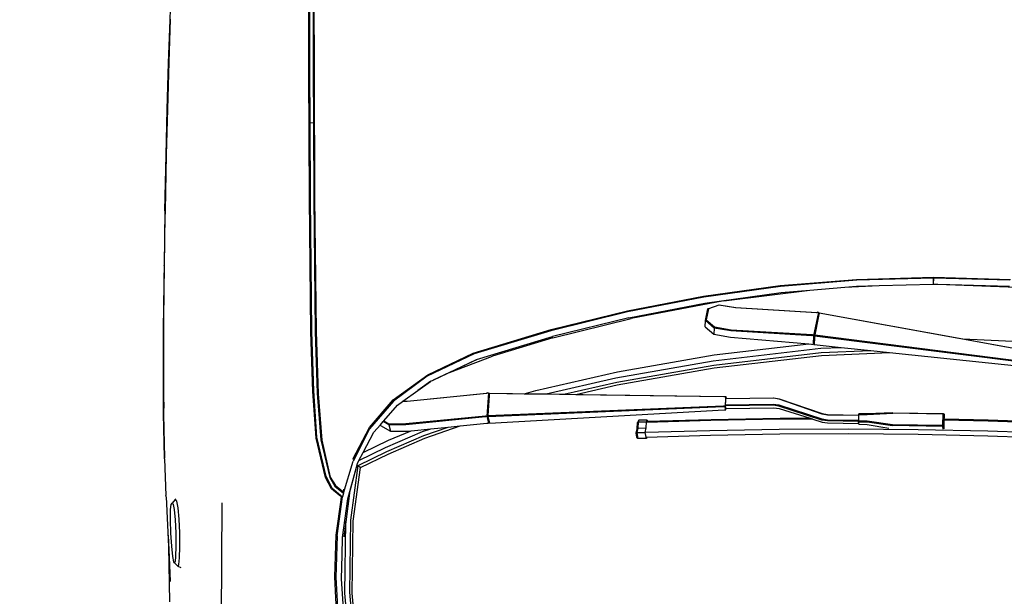
# Model space of a CAD drawing. Units: inches. Extents: x 0 to 4258, y 0 to 3769.
# Tile 12 of 30: x 3726 to 3763, y 3082 to 3104. Entities that reach past the tile are written whole.
import ezdxf

# ---------------------------------------------------------------- set-up
doc = ezdxf.new("R2010")
doc.units = ezdxf.units.IN
doc.header["$MEASUREMENT"] = 0
doc.layers.get('0').update_dxf_attribs({"color": 16})
doc.layers.add('A-ANNO-DIMS', color=250, linetype='Continuous', lineweight=18)
doc.layers.add('C-PKNG-VEHI', color=8, linetype='Continuous', lineweight=18)
doc.layers.add('Edges', color=250, linetype='Continuous')
doc.styles.get("Standard").update_dxf_attribs({"font": 'arial.ttf'})
doc.dimstyles.get("Standard").update_dxf_attribs({"dimtxt": 7, "dimasz": 0.18, "dimexe": 0.18, "dimexo": 0.0625, "dimgap": 0.09, "dimtad": 0, "dimtih": 1, "dimtoh": 1, "dimzin": 0, "dimdsep": 46, "dimlunit": 3, "dimtxsty": 'Standard', "dimcen": 0.09, "dimadec": 0, "dimazin": 0, "dimtfac": 1, "dimtofl": 0, "dimtmove": 0, "dimatfit": 3, "dimfxl": 1, "dimtolj": 1, "dimtzin": 0, "dimarcsym": 0})

# ---------------------------------------------------------------- blocks, each defined once
blk = doc.blocks.new('Nissan Qashqai pl')
at = {"layer": 'Edges'}
for p, q in [((8.4387, 12.0674), (8.4359, 11.9861)), ((8.4397, 12.0674), (8.4369, 11.9861)), ((8.4517, 12.0674), (8.4489, 11.9858)), ((8.4541, 11.9857), (8.4568, 12.0669)), ((8.3575, 12.0475), (8.3104, 11.7881)), ((8.3406, 11.9567), (8.3448, 12.0536)), ((8.3565, 11.8707), (8.3746, 12.0435)), ((8.336, 11.7828), (8.3688, 12.0419)), ((8.3702, 12.0427), (8.3374, 11.7826)), ((8.2765, 11.9273), (8.2804, 12.0305)), ((8.2682, 11.9221), (8.2708, 12.0123)), ((8.2719, 12.0118), (8.2695, 11.9221)), ((8.2765, 11.9273), (8.2788, 12.0114)), ((8.3406, 11.9567), (8.3495, 12.0053)), ((8.4359, 11.9861), (8.4348, 11.9346)), ((8.4369, 11.9861), (8.4358, 11.9346)), ((8.4489, 11.9858), (8.4471, 11.9043)), ((8.4523, 11.9043), (8.4541, 11.9857)), ((8.31, 11.7882), (8.3406, 11.9567)), ((8.4272, 11.8746), (8.4281, 11.9336)), ((8.4287, 11.9335), (8.4278, 11.8745)), ((8.4281, 11.9336), (8.429, 11.9345)), ((8.4281, 11.9336), (8.4287, 11.9336)), ((8.4287, 11.9335), (8.4281, 11.9336)), ((8.429, 11.9345), (8.4287, 11.9336)), ((8.4287, 11.9336), (8.4287, 11.9335)), ((8.4418, 11.9332), (8.4287, 11.9335)), ((8.4328, 11.9347), (8.429, 11.9345)), ((8.429, 11.9345), (8.4326, 11.9345)), ((8.4328, 11.9347), (8.4326, 11.9345)), ((8.4326, 11.9345), (8.4348, 11.9344)), ((8.4348, 11.9346), (8.4328, 11.9347)), ((8.4348, 11.9346), (8.4348, 11.9344)), ((8.4358, 11.9346), (8.4348, 11.9346)), ((8.4348, 11.9344), (8.4358, 11.9344)), ((8.4358, 11.9346), (8.4358, 11.9344)), ((8.4459, 11.9344), (8.4358, 11.9346)), ((8.4358, 11.9344), (8.4422, 11.9342)), ((8.441, 11.8742), (8.4418, 11.9332)), ((8.4418, 11.9332), (8.4422, 11.9342)), ((8.4431, 11.9332), (8.4418, 11.9332)), ((8.4422, 11.9342), (8.4459, 11.9344)), ((8.4422, 11.9342), (8.4431, 11.9332)), ((8.4431, 11.9332), (8.4422, 11.8742)), ((8.4464, 11.9334), (8.4431, 11.9332)), ((8.4459, 11.9344), (8.4459, 11.9344)), ((8.2708, 11.8319), (8.2682, 11.9221)), ((8.2763, 11.9223), (8.2695, 11.9221)), ((8.2695, 11.9221), (8.2763, 11.9219)), ((8.2695, 11.9221), (8.2719, 11.8323)), ((8.2763, 11.9223), (8.2764, 11.9263)), ((8.2763, 11.9219), (8.2763, 11.9223)), ((8.2781, 11.8585), (8.2763, 11.9219)), ((8.2764, 11.9263), (8.2765, 11.9273)), ((8.4471, 11.9043), (8.4464, 11.8227)), ((8.4516, 11.823), (8.4523, 11.9043)), ((8.3542, 11.8485), (8.3565, 11.8707)), ((8.3599, 11.7906), (8.3565, 11.8707)), ((8.4272, 11.8746), (8.4286, 11.8445)), ((8.4292, 11.8445), (8.4278, 11.8745)), ((8.4368, 11.8443), (8.441, 11.8742)), ((8.438, 11.8443), (8.4422, 11.8742)), ((8.28, 11.818), (8.2781, 11.8585)), ((8.2788, 11.8327), (8.2781, 11.8585)), ((8.2789, 11.8319), (8.2781, 11.8585)), ((8.4408, 11.8444), (8.4452, 11.8698)), ((8.3505, 11.8139), (8.3542, 11.8485)), ((8.3567, 11.7903), (8.3542, 11.8485)), ((8.4286, 11.8445), (8.4285, 11.8345)), ((8.4291, 11.8345), (8.4292, 11.8445)), ((8.4366, 11.8345), (8.4368, 11.8443)), ((8.4379, 11.8345), (8.438, 11.8443)), ((8.4406, 11.8344), (8.4408, 11.8444)), ((8.2781, 11.7423), (8.2708, 11.8319)), ((8.2719, 11.8323), (8.2793, 11.7426)), ((8.2789, 11.8319), (8.2788, 11.8327)), ((8.28, 11.818), (8.2789, 11.8319)), ((8.4291, 11.8345), (8.4285, 11.8345)), ((8.4298, 11.8345), (8.4291, 11.8345)), ((8.4292, 11.7978), (8.4298, 11.8345)), ((8.4304, 11.8345), (8.4298, 11.7978)), ((8.4304, 11.8345), (8.4298, 11.8345)), ((8.436, 11.8344), (8.4304, 11.8345)), ((8.4355, 11.7977), (8.436, 11.8344)), ((8.4366, 11.8343), (8.436, 11.8344)), ((8.4366, 11.8345), (8.4379, 11.8345)), ((8.4366, 11.8344), (8.4366, 11.8345)), ((8.4373, 11.8344), (8.4366, 11.8344)), ((8.4373, 11.8344), (8.4366, 11.8343)), ((8.4366, 11.8343), (8.4366, 11.8344)), ((8.4373, 11.8344), (8.4367, 11.7977)), ((8.4379, 11.8344), (8.4373, 11.8344)), ((8.4379, 11.8343), (8.4373, 11.8344)), ((8.4379, 11.8344), (8.4379, 11.8345)), ((8.4397, 11.8344), (8.4379, 11.8343)), ((8.4379, 11.8343), (8.4379, 11.8344)), ((8.4391, 11.7978), (8.4397, 11.8344)), ((8.4406, 11.8344), (8.4397, 11.8344)), ((8.2834, 11.7773), (8.28, 11.818)), ((8.3472, 11.7821), (8.3505, 11.8139)), ((8.3516, 11.79), (8.3505, 11.8139)), ((8.4464, 11.8227), (8.4468, 11.7413)), ((8.452, 11.7418), (8.4516, 11.823)), ((8.3662, 11.6639), (8.3516, 11.79)), ((8.3713, 11.6645), (8.3567, 11.7903)), ((8.3745, 11.665), (8.3599, 11.7906)), ((8.4107, 11.7411), (8.4281, 11.7914)), ((8.4287, 11.7914), (8.4111, 11.741)), ((8.4179, 11.7406), (8.4344, 11.7912)), ((8.4357, 11.7912), (8.4193, 11.7407)), ((8.4281, 11.7914), (8.4292, 11.7978)), ((8.4298, 11.7978), (8.4287, 11.7914)), ((8.4344, 11.7912), (8.4355, 11.7977)), ((8.4347, 11.7805), (8.4381, 11.7914)), ((8.4367, 11.7977), (8.4357, 11.7912)), ((8.4381, 11.7914), (8.4391, 11.7978)), ((8.3038, 11.6903), (8.3095, 11.7853)), ((8.3099, 11.7851), (8.3042, 11.6901)), ((8.3092, 11.7863), (8.3093, 11.7873)), ((8.3092, 11.7863), (8.3099, 11.7851)), ((8.3095, 11.7853), (8.3092, 11.7863)), ((8.3093, 11.7873), (8.3367, 11.7816)), ((8.3159, 11.7869), (8.3093, 11.7873)), ((8.31, 11.7882), (8.3104, 11.7881)), ((8.3104, 11.7881), (8.3159, 11.7869)), ((8.3159, 11.7869), (8.336, 11.7828)), ((8.3298, 11.6848), (8.3355, 11.7798)), ((8.3369, 11.7796), (8.3312, 11.6846)), ((8.3355, 11.7798), (8.3366, 11.7806)), ((8.336, 11.7828), (8.3374, 11.7826)), ((8.3367, 11.7816), (8.3366, 11.7806)), ((8.3366, 11.7806), (8.3369, 11.7796)), ((8.3367, 11.7816), (8.347, 11.7811)), ((8.3374, 11.7826), (8.3406, 11.7824)), ((8.3458, 11.7813), (8.3406, 11.7824)), ((8.3406, 11.7824), (8.3457, 11.7821)), ((8.3458, 11.7813), (8.3457, 11.7821)), ((8.3457, 11.7821), (8.3472, 11.7821)), ((8.347, 11.7811), (8.3458, 11.7813)), ((8.3464, 11.7761), (8.3467, 11.7791)), ((8.3467, 11.7791), (8.347, 11.7811)), ((8.4337, 11.7775), (8.4347, 11.7805)), ((8.4347, 11.7805), (8.4348, 11.7421)), ((8.296, 11.6762), (8.2834, 11.7773)), ((8.2862, 11.7434), (8.2834, 11.7773)), ((8.3385, 11.6842), (8.3464, 11.7761)), ((8.3593, 11.6651), (8.3464, 11.7761)), ((8.4222, 11.7413), (8.4337, 11.7775)), ((8.4337, 11.7775), (8.4339, 11.7423)), ((8.2985, 11.654), (8.2862, 11.7434)), ((8.2905, 11.6524), (8.2781, 11.7423)), ((8.2793, 11.7426), (8.2916, 11.6528)), ((8.4097, 11.7348), (8.4107, 11.7411)), ((8.4104, 11.6791), (8.4097, 11.7348)), ((8.4111, 11.741), (8.41, 11.7346)), ((8.41, 11.7346), (8.4108, 11.6791)), ((8.417, 11.7342), (8.4179, 11.7406)), ((8.4177, 11.678), (8.417, 11.7342)), ((8.4193, 11.7407), (8.4183, 11.7343)), ((8.4183, 11.7343), (8.4191, 11.678)), ((8.4213, 11.735), (8.4222, 11.7413)), ((8.4221, 11.6787), (8.4213, 11.735)), ((8.4339, 11.7423), (8.4353, 11.6613)), ((8.4348, 11.7421), (8.4362, 11.661)), ((8.4468, 11.7413), (8.4482, 11.66)), ((8.4534, 11.6608), (8.452, 11.7418)), ((8.3005, 11.6706), (8.3038, 11.6903)), ((8.3042, 11.6901), (8.3009, 11.6704)), ((8.296, 11.6762), (8.3166, 11.5675)), ((8.3264, 11.6652), (8.3298, 11.6848)), ((8.3312, 11.6846), (8.3278, 11.665)), ((8.3352, 11.6646), (8.3385, 11.6842)), ((8.4086, 11.6764), (8.4045, 11.4011)), ((8.4056, 11.5028), (8.4082, 11.6766)), ((8.4082, 11.6785), (8.4104, 11.6791)), ((8.4082, 11.6785), (8.4086, 11.6784)), ((8.4082, 11.6766), (8.4082, 11.6785)), ((8.4086, 11.6784), (8.4086, 11.6764)), ((8.4086, 11.6784), (8.4117, 11.6782)), ((8.4104, 11.6791), (8.4108, 11.6791)), ((8.4104, 11.6786), (8.4104, 11.6791)), ((8.4108, 11.6786), (8.4104, 11.6786)), ((8.4104, 11.6786), (8.4108, 11.6784)), ((8.4108, 11.6791), (8.4108, 11.6786)), ((8.4108, 11.6786), (8.4108, 11.6784)), ((8.4108, 11.6784), (8.4117, 11.6783)), ((8.4117, 11.6783), (8.4117, 11.6782)), ((8.4117, 11.6783), (8.4177, 11.678)), ((8.4117, 11.6782), (8.419, 11.6778)), ((8.4177, 11.678), (8.4191, 11.678)), ((8.419, 11.6778), (8.4203, 11.6778)), ((8.419, 11.6758), (8.419, 11.6778)), ((8.4305, 11.3996), (8.419, 11.6758)), ((8.4191, 11.678), (8.4221, 11.6787)), ((8.4238, 11.6786), (8.4203, 11.6778)), ((8.4203, 11.6778), (8.4204, 11.6758)), ((8.4204, 11.6758), (8.4319, 11.3996)), ((8.4238, 11.6786), (8.4221, 11.6787)), ((8.4238, 11.6766), (8.4238, 11.6786)), ((8.4394, 11.4014), (8.4238, 11.6766)), ((8.3053, 11.6574), (8.3005, 11.6706)), ((8.3009, 11.6704), (8.3054, 11.6583)), ((8.3182, 11.6557), (8.3264, 11.6652)), ((8.3278, 11.665), (8.319, 11.6546)), ((8.3264, 11.6542), (8.3352, 11.6646)), ((8.3278, 11.665), (8.3352, 11.6646)), ((8.3792, 11.5515), (8.3593, 11.6651)), ((8.3864, 11.5497), (8.3662, 11.6639)), ((8.3913, 11.5506), (8.3713, 11.6645)), ((8.3945, 11.5513), (8.3745, 11.665)), ((8.3076, 11.5631), (8.2905, 11.6524)), ((8.2916, 11.6528), (8.3089, 11.5631)), ((8.3157, 11.5647), (8.2985, 11.654)), ((8.3054, 11.6583), (8.3053, 11.6574)), ((8.319, 11.6546), (8.3053, 11.6574)), ((8.3054, 11.6583), (8.3182, 11.6557)), ((8.319, 11.6546), (8.3182, 11.6557)), ((8.3264, 11.6542), (8.319, 11.6546)), ((8.4353, 11.6613), (8.4375, 11.5863)), ((8.4362, 11.661), (8.4385, 11.5858)), ((8.4482, 11.66), (8.4505, 11.5843)), ((8.4557, 11.5855), (8.4534, 11.6608)), ((8.4377, 11.5857), (8.4357, 11.5864)), ((8.4357, 11.5864), (8.4359, 11.5765)), ((8.4357, 11.5864), (8.4375, 11.5863)), ((8.4375, 11.5863), (8.4375, 11.5862)), ((8.4379, 11.5758), (8.4377, 11.5857)), ((8.445, 11.5853), (8.4377, 11.5857)), ((8.4452, 11.5754), (8.445, 11.5853)), ((8.4503, 11.5841), (8.445, 11.5853)), ((8.4572, 11.5854), (8.4503, 11.5841)), ((8.4505, 11.5742), (8.4503, 11.5841)), ((8.4557, 11.5855), (8.4572, 11.5854)), ((8.4557, 11.5853), (8.4557, 11.5855)), ((8.4572, 11.5854), (8.4574, 11.5755)), ((8.4359, 11.5765), (8.4379, 11.5758)), ((8.4359, 11.5765), (8.4377, 11.5753)), ((8.4387, 11.5749), (8.4377, 11.5753)), ((8.4379, 11.5758), (8.4452, 11.5754)), ((8.4384, 11.5752), (8.4457, 11.5749)), ((8.446, 11.5746), (8.4387, 11.5749)), ((8.4452, 11.5754), (8.4505, 11.5742)), ((8.4507, 11.5734), (8.446, 11.5746)), ((8.4505, 11.5742), (8.4574, 11.5755)), ((8.4507, 11.5734), (8.4505, 11.5742)), ((8.4559, 11.5744), (8.4507, 11.5734)), ((8.4574, 11.5755), (8.4559, 11.5744)), ((8.3296, 11.4739), (8.3076, 11.5631)), ((8.3089, 11.5631), (8.3311, 11.4733)), ((8.3157, 11.5647), (8.3377, 11.4753)), ((8.3392, 11.4758), (8.3166, 11.5675)), ((8.4009, 11.4559), (8.3792, 11.5515)), ((8.4051, 11.4678), (8.3864, 11.5497)), ((8.4054, 11.4887), (8.3913, 11.5506)), ((8.4056, 11.5028), (8.3945, 11.5513)), ((8.4054, 11.4887), (8.4056, 11.5028)), ((8.4051, 11.4678), (8.4054, 11.4887)), ((8.3573, 11.3824), (8.3296, 11.4739)), ((8.3311, 11.4733), (8.3582, 11.3836)), ((8.3648, 11.3863), (8.3377, 11.4753)), ((8.3392, 11.4758), (8.3608, 11.4048)), ((8.4048, 11.4423), (8.4051, 11.4678)), ((8.4048, 11.4423), (8.4009, 11.4559)), ((8.4041, 11.4013), (8.4048, 11.4423)), ((8.3799, 11.3545), (8.3608, 11.4048)), ((8.407, 11.401), (8.4037, 11.4002)), ((8.4037, 11.4002), (8.4314, 11.3985)), ((8.4037, 11.3992), (8.4037, 11.4002)), ((8.4037, 11.3992), (8.4046, 11.3981)), ((8.4042, 11.3983), (8.4037, 11.3992)), ((8.4041, 11.4013), (8.4045, 11.4011)), ((8.4134, 11.3049), (8.4042, 11.3983)), ((8.4045, 11.4011), (8.407, 11.401)), ((8.4046, 11.3981), (8.4138, 11.3048)), ((8.407, 11.401), (8.4305, 11.3996)), ((8.4305, 11.3996), (8.4319, 11.3996)), ((8.4306, 11.3966), (8.4314, 11.3975)), ((8.4398, 11.3032), (8.4306, 11.3966)), ((8.4314, 11.3985), (8.4394, 11.4004)), ((8.4314, 11.3985), (8.4314, 11.3975)), ((8.4314, 11.3975), (8.4319, 11.3967)), ((8.4319, 11.3996), (8.436, 11.4006)), ((8.4319, 11.3967), (8.4412, 11.3033)), ((8.436, 11.4006), (8.4394, 11.4014)), ((8.4394, 11.4004), (8.436, 11.4006)), ((8.4394, 11.3984), (8.4394, 11.4004)), ((8.4425, 11.3672), (8.4394, 11.3984)), ((8.3646, 11.387), (8.3799, 11.3545)), ((8.3888, 11.3355), (8.3648, 11.3863)), ((8.3826, 11.3291), (8.3573, 11.3824)), ((8.3582, 11.3836), (8.3844, 11.3284)), ((8.4571, 11.3258), (8.4425, 11.3672)), ((8.4439, 11.3531), (8.4425, 11.3672)), ((8.3799, 11.3545), (8.3888, 11.3355)), ((8.454, 11.3245), (8.4439, 11.3531)), ((8.4459, 11.3326), (8.4439, 11.3531)), ((8.4122, 11.2883), (8.3826, 11.3291)), ((8.3844, 11.3284), (8.4134, 11.2888)), ((8.3901, 11.3328), (8.3888, 11.3355)), ((8.3901, 11.3328), (8.4011, 11.3173)), ((8.3904, 11.3321), (8.3901, 11.3328)), ((8.4011, 11.3173), (8.3904, 11.3321)), ((8.4493, 11.3229), (8.4459, 11.3326)), ((8.4482, 11.3095), (8.4459, 11.3326)), ((8.4135, 11.3), (8.4011, 11.3173)), ((8.468, 11.2793), (8.4493, 11.3229)), ((8.4725, 11.2812), (8.454, 11.3245)), ((8.4756, 11.2826), (8.4571, 11.3258)), ((8.4135, 11.3), (8.4134, 11.3049)), ((8.4138, 11.3048), (8.4139, 11.2994)), ((8.4594, 11.2831), (8.4482, 11.3095)), ((8.4487, 11.305), (8.4482, 11.3095)), ((8.4489, 11.2852), (8.4487, 11.305)), ((8.4139, 11.2994), (8.4135, 11.3)), ((8.4183, 11.2934), (8.4139, 11.2994)), ((8.4365, 11.2776), (8.4183, 11.2934)), ((8.44, 11.2834), (8.4398, 11.3032)), ((8.4412, 11.3033), (8.4415, 11.2835)), ((8.4444, 11.2608), (8.4122, 11.2883)), ((8.4134, 11.2888), (8.4462, 11.2609)), ((8.4365, 11.2776), (8.44, 11.2834)), ((8.4415, 11.2835), (8.4375, 11.2767)), ((8.4415, 11.2835), (8.4489, 11.2852)), ((8.4422, 11.2737), (8.4489, 11.2852)), ((8.4737, 11.2534), (8.4594, 11.2831)), ((8.4889, 11.2473), (8.4725, 11.2812)), ((8.4914, 11.25), (8.4756, 11.2826)), ((8.4375, 11.2767), (8.4365, 11.2776)), ((8.4412, 11.2735), (8.4375, 11.2767)), ((8.4422, 11.2737), (8.4412, 11.2735)), ((8.4499, 11.2659), (8.4412, 11.2735)), ((8.4831, 11.2484), (8.468, 11.2793)), ((8.4814, 11.2413), (8.4444, 11.2608)), ((8.4462, 11.2609), (8.4838, 11.2415)), ((8.4737, 11.2534), (8.4499, 11.2659)), ((8.4831, 11.2484), (8.4737, 11.2534)), ((8.4867, 11.2465), (8.4831, 11.2484)), ((8.528, 11.2354), (8.4867, 11.2465)), ((8.5214, 11.2374), (8.4867, 11.2465)), ((8.4889, 11.2473), (8.4914, 11.25)), ((8.5531, 11.2387), (8.4889, 11.2473)), ((8.5544, 11.2416), (8.4914, 11.25)), ((8.7481, 11.2473), (8.6375, 11.2376)), ((8.7491, 11.2501), (8.6386, 11.2404)), ((8.5216, 11.2303), (8.4838, 11.2415)), ((8.5214, 11.2374), (8.555, 11.233)), ((8.5301, 11.2352), (8.5214, 11.2374)), ((8.5736, 11.2291), (8.528, 11.2354)), ((8.6375, 11.2376), (8.5531, 11.2387)), ((8.6386, 11.2404), (8.5544, 11.2416)), ((8.5125, 11.221), (8.5177, 11.2272)), ((8.5132, 11.2202), (8.5216, 11.2303)), ((8.5155, 11.2168), (8.5258, 11.2291)), ((8.5237, 11.2252), (8.5163, 11.2162)), ((8.5197, 11.2297), (8.5166, 11.2307)), ((8.5177, 11.2272), (8.5197, 11.2297)), ((8.5216, 11.2303), (8.5197, 11.2297)), ((8.5216, 11.2303), (8.5258, 11.2291)), ((8.5259, 11.2279), (8.5237, 11.2252)), ((8.5258, 11.2291), (8.5259, 11.2279)), ((8.5715, 11.2227), (8.5258, 11.2291)), ((8.5294, 11.2274), (8.5259, 11.2279)), ((8.5706, 11.2216), (8.5294, 11.2274)), ((8.6387, 11.2319), (8.555, 11.233)), ((8.555, 11.233), (8.5726, 11.2307)), ((8.5941, 11.2286), (8.5736, 11.2291)), ((8.5941, 11.2289), (8.5941, 11.2286)), ((8.622, 11.228), (8.5941, 11.2286)), ((8.6203, 11.2213), (8.6721, 11.2241)), ((8.6699, 11.231), (8.622, 11.228)), ((8.6721, 11.2348), (8.6387, 11.2319)), ((8.4588, 11.2036), (8.5032, 11.2141)), ((8.4595, 11.2047), (8.5025, 11.2148)), ((8.5155, 11.2168), (8.5018, 11.2098)), ((8.5025, 11.2148), (8.5125, 11.221)), ((8.5163, 11.2162), (8.5029, 11.2092)), ((8.5032, 11.2141), (8.5132, 11.2202)), ((8.6197, 11.2201), (8.5706, 11.2216)), ((8.5715, 11.2227), (8.6203, 11.2213)), ((8.6683, 11.2226), (8.6197, 11.2201)), ((8.3318, 11.198), (8.4049, 11.2004)), ((8.4042, 11.1995), (8.4588, 11.2036)), ((8.4049, 11.2004), (8.4595, 11.2047)), ((8.5018, 11.2098), (8.4559, 11.1991)), ((8.5029, 11.2092), (8.4571, 11.1983)), ((8.0276, 11.1896), (7.904, 11.1894)), ((8.0275, 11.1909), (7.9176, 11.1908)), ((7.9183, 11.1947), (8.0275, 11.1948)), ((7.9185, 11.1955), (8.0273, 11.1957)), ((8.0273, 11.1957), (8.1753, 11.1963)), ((8.0275, 11.1948), (8.0876, 11.1951)), ((8.0873, 11.1911), (8.0275, 11.1909)), ((8.1753, 11.1903), (8.0276, 11.1896)), ((8.0876, 11.1951), (8.0873, 11.1911)), ((8.1755, 11.1915), (8.0873, 11.1911)), ((8.0876, 11.1951), (8.1754, 11.1954)), ((8.1753, 11.1963), (8.3318, 11.198)), ((8.3324, 11.192), (8.1753, 11.1903)), ((8.1754, 11.1954), (8.332, 11.1971)), ((8.3324, 11.1931), (8.1755, 11.1915)), ((8.332, 11.1971), (8.4042, 11.1995)), ((8.4014, 11.1953), (8.3324, 11.1931)), ((8.4022, 11.1943), (8.3324, 11.192)), ((8.4559, 11.1991), (8.4014, 11.1953)), ((8.4571, 11.1983), (8.4022, 11.1943)), ((8.5326, 11.0874), (8.6675, 11.0866)), ((8.609, 11.0397), (8.6073, 11.0362)), ((7.9668, 11.0268), (7.9151, 11.029)), ((8.5283, 11.0336), (8.5287, 11.0329)), ((8.531, 11.0346), (8.5287, 11.0329)), ((8.5287, 11.0329), (8.5331, 11.0292)), ((8.5385, 11.0363), (8.531, 11.0346)), ((8.5331, 11.0292), (8.5346, 11.0303)), ((8.5347, 11.0282), (8.5331, 11.0292)), ((8.5346, 11.0303), (8.5406, 11.0316)), ((8.5407, 11.0274), (8.5347, 11.0282)), ((8.5518, 11.0375), (8.5385, 11.0363)), ((8.5406, 11.0316), (8.5526, 11.0328)), ((8.5527, 11.0273), (8.5407, 11.0274)), ((8.568, 11.0382), (8.5518, 11.0375)), ((8.5526, 11.0328), (8.5681, 11.0335)), ((8.5682, 11.0278), (8.5527, 11.0273)), ((8.5842, 11.0384), (8.568, 11.0382)), ((8.5681, 11.0335), (8.5836, 11.0337)), ((8.5837, 11.0288), (8.5682, 11.0278)), ((8.5836, 11.0337), (8.5957, 11.0334)), ((8.5958, 11.0301), (8.5837, 11.0288)), ((8.5974, 11.0381), (8.5842, 11.0384)), ((8.5957, 11.0334), (8.6017, 11.0328)), ((8.6018, 11.0312), (8.5958, 11.0301)), ((8.6049, 11.0373), (8.5974, 11.0381)), ((8.6017, 11.0328), (8.6032, 11.0321)), ((8.6032, 11.0321), (8.6018, 11.0312)), ((8.6073, 11.0362), (8.6032, 11.0321)), ((8.6073, 11.0362), (8.6049, 11.0373)), ((7.9658, 11.027), (8.016, 11.0253)), ((8.0168, 11.0251), (7.9668, 11.0268)), ((8.016, 11.0253), (8.0713, 11.0237)), ((8.0718, 11.0235), (8.0168, 11.0251)), ((8.0713, 11.0237), (8.1249, 11.0223)), ((8.1251, 11.0222), (8.0718, 11.0235)), ((8.1249, 11.0223), (8.1901, 11.021)), ((8.1902, 11.0208), (8.1251, 11.0222)), ((8.1901, 11.021), (8.1938, 11.021)), ((8.1902, 11.021), (8.1938, 11.021)), ((8.1904, 11.0209), (8.1902, 11.0208)), ((8.1904, 11.0209), (8.2543, 11.0198)), ((8.1938, 11.021), (8.1954, 11.0209)), ((8.1954, 11.0209), (8.2544, 11.02)), ((8.2544, 11.0198), (8.2543, 11.0199)), ((8.2543, 11.0198), (8.2544, 11.0198)), ((8.2544, 11.02), (8.3166, 11.0193)), ((8.2544, 11.0198), (8.2556, 11.0198)), ((8.2556, 11.0198), (8.256, 11.0198)), ((8.256, 11.0198), (8.2561, 11.0198)), ((8.2561, 11.0198), (8.2693, 11.0197)), ((8.2693, 11.0197), (8.2694, 11.0197)), ((8.2694, 11.0197), (8.3098, 11.0192)), ((8.3098, 11.0192), (8.3163, 11.0192)), ((8.3663, 11.019), (8.3163, 11.0192)), ((8.3597, 11.019), (8.3163, 11.0192)), ((8.3166, 11.0193), (8.3764, 11.0191)), ((8.3602, 11.019), (8.3597, 11.019)), ((8.3608, 11.019), (8.3602, 11.019)), ((8.3663, 11.019), (8.3608, 11.019)), ((8.3663, 11.019), (8.3764, 11.0191)), ((8.3757, 11.019), (8.3663, 11.019)), ((8.4282, 11.0193), (8.3757, 11.019)), ((8.3764, 11.0191), (8.4069, 11.0192)), ((8.4069, 11.0192), (8.4219, 11.0196)), ((8.4069, 11.0192), (8.4292, 11.0193)), ((8.4799, 11.0202), (8.4282, 11.0193)), ((8.4292, 11.0193), (8.4799, 11.0202)), ((8.4811, 11.0203), (8.4799, 11.0202)), ((8.4811, 11.0203), (8.5241, 11.022)), ((8.5259, 11.0221), (8.5241, 11.022)), ((8.5259, 11.0221), (8.5838, 11.0251)), ((8.5707, 11.0248), (8.5965, 11.0258)), ((8.5838, 11.0251), (8.6489, 11.0263)), ((8.5838, 11.0251), (8.5965, 11.0258)), ((8.5965, 11.0258), (8.6252, 11.0268))]:
    blk.add_line(p, q, dxfattribs=at)
blk = doc.blocks.new('car')
blk.add_blockref('Nissan Qashqai pl', (-9.7433, -11.9151))
blk = doc.blocks.new('*D66')
at = {"layer": 'A-ANNO-DIMS', "color": 0, "lineweight": -2, "transparency": 16777216}
for p, q in [((3725.517, 3125.846), (3703.936, 3125.846)), ((3704.116, 3125.666), (3704.116, 3058.01)), ((3704.116, 2982.935), (3704.116, 3050.591)), ((3725.517, 2982.755), (3703.936, 2982.755))]:
    blk.add_line(p, q, dxfattribs=at)
at = {"layer": 'A-ANNO-DIMS', "color": 0, "transparency": 16777216}
for points in [[(3704.086, 3125.666), (3704.146, 3125.666), (3704.116, 3125.846)], [(3704.086, 2982.935), (3704.146, 2982.935), (3704.116, 2982.755)]]:
    blk.add_solid(points, dxfattribs=at)
at = {"layer": 'Defpoints', "color": 0, "transparency": 16777216}
for p in [(3725.58, 3125.846), (3704.116, 2982.755), (3725.58, 2982.755)]:
    blk.add_point(p, dxfattribs=at)
at = {"layer": 'A-ANNO-DIMS', "color": 0, "transparency": 16777216, "insert": (3704.116, 3054.301), "char_height": 7, "attachment_point": 5}
blk.add_mtext('\\A1;CAR 11\'-11"', dxfattribs=at)

msp = doc.modelspace()

# ---------------------------------------------------------------- block references
at = {"layer": 'C-PKNG-VEHI', "xscale": 32.66500240257601, "yscale": 32.66500240257601, "zscale": 32.66500240257601, "rotation": 270}
msp.add_blockref('car', (3760.419, 3045.57), dxfattribs=at)

# ---------------------------------------------------------------- dimensions: what is measured, and where the dimension line sits
at = {"layer": 'A-ANNO-DIMS'}
dim = msp.add_linear_dim(base=(3704.116, 2982.755), p1=(3725.58, 3125.846), p2=(3725.58, 2982.755), angle=270, text='CAR <>', dimstyle='Standard', override={"dimdec": 1, "dimlfac": 1, "dimrnd": 0, "dimzin": 1, "dimdsep": 46, "dimlunit": 4, "dimfrac": 2}, dxfattribs=at)
dim.commit()
dim.dimension.update_dxf_attribs({"geometry": '*D66', "text_midpoint": (3704.116, 3054.301)})

doc.saveas('drawing.dxf')
